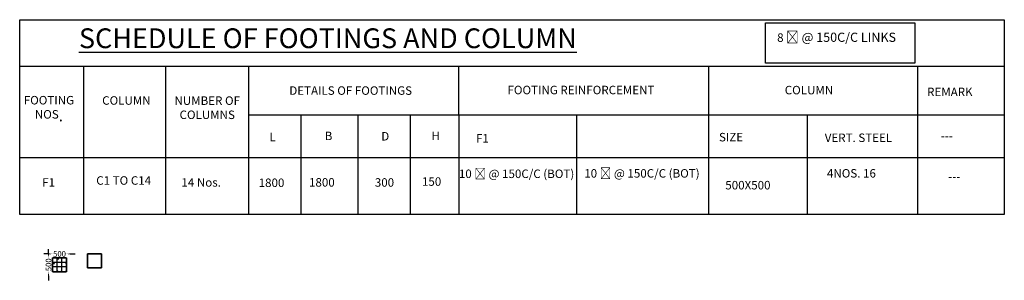
# Model space of a CAD drawing. Units: millimetres. Extents: x -106221 to -52078, y 251365 to 289027.
# Tile 2 of 2: x -86862 to -52078, y 279810 to 289027. Entities that reach past the tile are written whole.
import ezdxf

# ---------------------------------------------------------------- set-up
doc = ezdxf.new("R2010")
doc.units = ezdxf.units.MM
doc.header["$LTSCALE"] = 15
doc.header["$MEASUREMENT"] = 0
for name, color, linetype, lineweight in [('S-ANNO-DIMS', 2, 'Continuous', 18), ('S-ANNO-SCHD', 7, 'Continuous', 25), ('S-ANNO-TEXT', 7, 'Continuous', 25), ('S-COLS', 1, 'Continuous', 35), ('S-REIN', 1, 'Continuous', 25)]:
    doc.layers.add(name, color=color, linetype=linetype, lineweight=lineweight)
doc.styles.get("Standard").update_dxf_attribs({"font": 'arial.ttf'})
doc.dimstyles.get("Standard").update_dxf_attribs({"dimtxt": 200, "dimasz": 150, "dimexe": 0.18, "dimexo": 0.0625, "dimgap": 0.09, "dimtad": 0, "dimdec": 0, "dimzin": 0, "dimdsep": 46, "dimtxsty": 'Standard', "dimcen": 0.09, "dimadec": 0, "dimazin": 0, "dimtfac": 1, "dimtdec": 0, "dimtofl": 0, "dimtmove": 0, "dimatfit": 3, "dimfxl": 1, "dimfxlon": 1, "dimtolj": 1, "dimtzin": 0, "dimarcsym": 0})

# ---------------------------------------------------------------- blocks, each defined once
blk = doc.blocks.new('*D10')
at = {"layer": 'Defpoints', "color": 0, "ltscale": 15, "transparency": 16777216}
for p in [(-85205, 280743), (-85705, 280539), (-85205, 280539)]:
    blk.add_point(p, dxfattribs=at)
at = {"layer": 'S-ANNO-DIMS', "color": 0, "lineweight": -2, "ltscale": 15, "transparency": 16777216}
for p, q in [((-85855, 280743), (-86005, 280743)), ((-85705, 280742), (-85705, 280743)), ((-85205, 280742), (-85205, 280743)), ((-85055, 280743), (-84905, 280743))]:
    blk.add_line(p, q, dxfattribs=at)
at = {"layer": 'S-ANNO-DIMS', "color": 0, "ltscale": 15, "transparency": 16777216}
for points in [[(-85855, 280768), (-85855, 280718), (-85705, 280743)], [(-85055, 280768), (-85055, 280718), (-85205, 280743)]]:
    blk.add_solid(points, dxfattribs=at)
at = {"layer": 'S-ANNO-DIMS', "color": 0, "ltscale": 15, "transparency": 16777216, "insert": (-85455, 280743), "char_height": 200, "attachment_point": 5}
blk.add_mtext('\\A1;500', dxfattribs=at)
blk = doc.blocks.new('*D11')
at = {"layer": 'Defpoints', "color": 0, "ltscale": 15, "transparency": 16777216}
for p in [(-85843, 280610), (-85616, 280610), (-85616, 280110)]:
    blk.add_point(p, dxfattribs=at)
at = {"layer": 'S-ANNO-DIMS', "color": 0, "lineweight": -2, "ltscale": 15, "transparency": 16777216}
for p, q in [((-85843, 280760), (-85843, 280910)), ((-85842, 280610), (-85843, 280610)), ((-85842, 280110), (-85843, 280110)), ((-85843, 279960), (-85843, 279810))]:
    blk.add_line(p, q, dxfattribs=at)
at = {"layer": 'S-ANNO-DIMS', "color": 0, "ltscale": 15, "transparency": 16777216}
for points in [[(-85868, 280760), (-85818, 280760), (-85843, 280610)], [(-85868, 279960), (-85818, 279960), (-85843, 280110)]]:
    blk.add_solid(points, dxfattribs=at)
at = {"layer": 'S-ANNO-DIMS', "color": 0, "ltscale": 15, "transparency": 16777216, "insert": (-85843, 280360), "char_height": 200, "attachment_point": 5, "rotation": 90}
blk.add_mtext('\\A1;500', dxfattribs=at)

msp = doc.modelspace()

# ---------------------------------------------------------------- linework, layer by layer
at = {"layer": 'S-ANNO-SCHD', "ltscale": 15}
for p, q in [((-86862.2, 287379.5), (-52077.6, 287379.5)), ((-84607.2, 287379.5), (-84607.2, 282140.4)), ((-81711.6, 287379.5), (-81711.6, 282140.4)), ((-78774, 287379.5), (-78774, 282140.4)), ((-71346.3, 285661.1), (-71346.3, 287379.5)), ((-62533.6, 287379.5), (-62533.6, 282140.4)), ((-55141.1, 287379.5), (-55141.1, 282140.4)), ((-78774, 285661.1), (-52077.6, 285661.1)), ((-76927.6, 285661.1), (-76927.6, 282140.4)), ((-74913.3, 285661.1), (-74913.3, 282140.4)), ((-73066.8, 285661.1), (-73066.8, 282140.4)), ((-71346.3, 285661.1), (-71346.3, 282140.4)), ((-67191.7, 285661.1), (-67191.7, 282140.4)), ((-59043.8, 285661.1), (-59043.8, 282140.4)), ((-86862.2, 284152.2), (-52077.6, 284152.2))]:
    msp.add_line(p, q, dxfattribs=at)
for points in [[(-86862.2, 289026.5), (-52077.6, 289026.5), (-52077.6, 282140.4), (-86862.2, 282140.4)], [(-60509.1, 288910.8), (-55233.2, 288910.8), (-55233.2, 287487), (-60509.1, 287487)]]:
    msp.add_lwpolyline(points, close=True, dxfattribs=at)
at = {"layer": 'S-COLS', "ltscale": 15}
msp.add_lwpolyline([(-84452.1, 280752.1), (-83992.1, 280752.1, -0.4142136), (-83972.1, 280732.1), (-83972.1, 280272.1, -0.4142136), (-83992.1, 280252.1), (-84452.1, 280252.1, -0.4142136), (-84472.1, 280272.1), (-84472.1, 280732.1, -0.4142136)], format="xyb", close=True, dxfattribs=at)
for points in [[(-85705.3, 280125.4), (-85705.3, 280595.5)], [(-85690.3, 280610.5), (-85220.2, 280610.5)], [(-85205.3, 280595.5), (-85205.3, 280125.4)], [(-85220.2, 280110.5), (-85690.3, 280110.5)]]:
    msp.add_lwpolyline(points, dxfattribs=at)
at = {"layer": 'S-REIN', "ltscale": 15}
for p, q in [((-85695.8, 280410), (-85646.6, 280390.5)), ((-85219.4, 280438.8), (-85691.1, 280438.8)), ((-85684.3, 280437.6), (-85635.4, 280416.3)), ((-85541.1, 280125.4), (-85541.1, 280595.5)), ((-85534.2, 280582.9), (-85495.4, 280558.3)), ((-85518.2, 280608.1), (-85479.4, 280583.4)), ((-85369.4, 280125.4), (-85369.4, 280595.5)), ((-85220.2, 280282.1), (-85690.3, 280282.1))]:
    msp.add_line(p, q, dxfattribs=at)
for centre in [(-85690.3, 280595.5), (-85690.3, 280423.9), (-85526.2, 280595.5), (-85384.3, 280595.5), (-85220.2, 280595.5), (-85220.2, 280423.9), (-85690.3, 280297), (-85690.3, 280125.4), (-85526.2, 280125.4), (-85384.3, 280125.4), (-85220.2, 280297), (-85220.2, 280125.4)]:
    msp.add_circle(centre, 14.9, dxfattribs=at)

# ---------------------------------------------------------------- texts
at = {"layer": 'S-ANNO-TEXT', "ltscale": 15, "attachment_point": 1}
for s, width, gutter_width, heights, insert, char_height in [('{\\fArial|b1|i0|c0|p34;\\LSCHEDULE OF FOOTINGS AND COLUMN}', 20064.272, 85.1, [262.2], (-84769, 288719.3), 700), ('8 {\\H1.08333x;ṓ @ 150C/C LINKS}', 4750.271, 1, [0], (-60102.3, 288567.1), 300), ('\\pxqc;{\\H0.75x;DETAILS OF FOOTINGS}', 7585.845, 1, [0], (-78961.7, 286669.7), 400), ('\\pxqc;{\\H0.75x;FOOTING REINFORCEMENT}', 9191.16, 1, [0], (-71629.3, 286689.8), 400), ('\\pxqc;{\\H0.75x;COLUMN}', 2727.658, 1, [0], (-60342.6, 286686.1), 400), ('\\pxqc;{\\H0.75x;FOOTING\\PNOS}.', 2727.658, 1, [0], (-87193.5, 286329.4), 400), ('\\pxqc;{\\H0.75x;COLUMN}', 2727.658, 1, [0], (-84455.5, 286319.4), 400), ('\\pxqc;{\\H0.75x;NUMBER OF COLUMNS}', 2727.658, 1, [0], (-81600.3, 286313.8), 400), ('{\\H0.75x;REMARK }', 2727.658, 1, [0], (-54805.3, 286622.8), 400), ('\\pxqc;{\\H0.75x;L}', 1018.729, 1, [0], (-78435.6, 285025.6), 400), ('\\pxqc;{\\H0.75x;B}', 1018.729, 1, [0], (-76460.8, 285066.7), 400), ('\\pxqc;{\\H0.75x;D}', 1018.729, 1, [0], (-74457.1, 285054.2), 400), ('\\pxqc;{\\H0.75x;H}', 1018.729, 1, [0], (-72674.2, 285067.9), 400), ('\\pxqc;{\\H0.75x;F1}', 1018.729, 1, [0], (-71023.4, 284982), 400), ('\\pxqc;{\\H0.75x;SIZE}', 1018.729, 1, [0], (-62241, 285022.8), 400), ('\\pxqc;{\\H0.75x;VERT. STEEL}', 3131.12, 1, [0], (-58796.5, 285000.7), 400), ('\\pxqc;{\\H0.75x;---}', 1018.729, 1, [0], (-54618.8, 285070.1), 400), ('{\\H0.75x;C1 TO C14}', 2315.693, 1, [0], (-84157.2, 283490.2), 400), ('10 ṓ @ 150C/C (BOT)', 5329.163, 1, [0], (-71346.3, 283727.7), 300), ('10 ṓ @ 150C/C (BOT)', 4396.85, 1, [0], (-66916.9, 283742.2), 300), ('\\pxqc;{\\H0.75x;4NOS. 16}', 2281.308, 1, [0], (-58619.7, 283743.6), 400), ('\\pxqc;{\\H0.75x;F1}', 1018.729, 1, [0], (-86351.4, 283421.7), 400), ('\\pxqc;{\\H0.75x;14 Nos.}', 1734.296, 1, [0], (-81318.3, 283421.7), 400), ('\\pxqc;{\\H0.75x;1800}', 1018.729, 1, [0], (-78475.3, 283410.5), 400), ('\\pxqc;{\\H0.75x;1800}', 1018.729, 1, [0], (-76696.7, 283424.2), 400), ('\\pxqc;{\\H0.75x;300}', 1018.729, 1, [0], (-74484.7, 283420.6), 400), ('\\pxqc;{\\H0.75x;150}', 1018.729, 1, [0], (-72819.1, 283453.4), 400), ('\\pxqc;{\\H0.75x;500X500}', 1989.943, 1, [0], (-62130.4, 283324.6), 400), ('\\pxqc;{\\H0.75x;---}', 1018.729, 1, [0], (-54353.1, 283632.5), 400)]:
    msp.add_mtext_dynamic_manual_height_columns(s, width=width, gutter_width=gutter_width, heights=heights, dxfattribs=dict(at, insert=insert, char_height=char_height))

# ---------------------------------------------------------------- dimensions: what is measured, and where the dimension line sits
at = {"layer": 'S-ANNO-DIMS', "ltscale": 15}
dim = msp.add_linear_dim(base=(-85205.3, 280743.3), p1=(-85705.3, 280539.1), p2=(-85205.3, 280539.1), dimstyle='Standard', override={"dimclrd": 0, "dimclre": 0, "dimclrt": 0}, dxfattribs=at)
dim.commit()
dim.dimension.update_dxf_attribs({"geometry": '*D10', "text_midpoint": (-85455.3, 280743.3)})
dim = msp.add_linear_dim(base=(-85842.6, 280610.5), p1=(-85616.3, 280110.5), p2=(-85616.3, 280610.5), angle=90, dimstyle='Standard', override={"dimclrd": 0, "dimclre": 0, "dimclrt": 0}, dxfattribs=at)
dim.commit()
dim.dimension.update_dxf_attribs({"geometry": '*D11', "text_midpoint": (-85842.6, 280360.5)})

doc.saveas('drawing.dxf')
